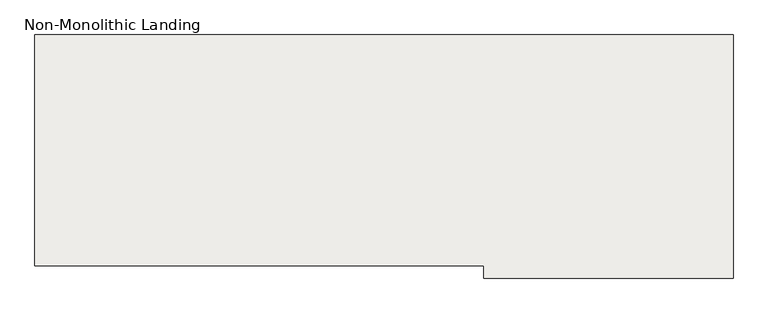
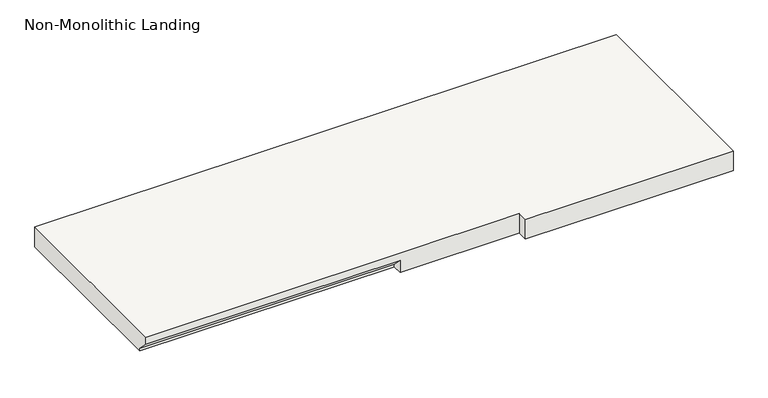
"""IFC4 building model written with IfcOpenShell, lengths in millimetres: slab geometry, Non-Monolithic Landing."""

from ifc_helpers import new_model, si_unit, origin, place, context, project, spatial, faceted_brep, source, transform, mapped, element, save


def non_monolithic_landing_1ef36e8a(model_context):
    return source(origin(), model_context, "Body", "Brep", [
        faceted_brep([(-1534.6629117, -2802.9424149, 1166.2833333), (-1534.6629117, -2777.5424149, 1140.8833333), (-912.3629117, -2777.5424149, 1140.8833333), (-912.3629117, -2802.9424149, 1166.2833333), (-620.2629117, -2802.9424149, 1185.3333333), (-620.2629117, -2828.3424149, 1185.3333333), (-112.2629117, -2828.3424149, 1185.3333333), (-112.2629117, -2802.9424149, 1185.3333333), (-112.2629117, -2333.0424149, 1185.3333333), (-1534.6629117, -2333.0424149, 1185.3333333), (-1534.6629117, -2802.9424149, 1185.3333333), (-912.3629117, -2777.5424149, 1134.5333333), (-1534.6629117, -2777.5424149, 1134.5333333), (-1534.6629117, -2333.0424149, 1134.5333333), (-112.2629117, -2333.0424149, 1134.5333333), (-112.2629117, -2802.9424149, 1134.5333333), (-112.2629117, -2828.3424149, 1134.5333333), (-620.2629117, -2828.3424149, 1134.5333333), (-620.2629117, -2802.9424149, 1134.5333333), (-912.3629117, -2802.9424149, 1134.5333333)], [[[0, 1, 2, 3]], [[4, 5, 6, 7, 8, 9, 10]], [[11, 12, 13, 14, 15, 16, 17, 18, 19]], [[12, 11, 2, 1]], [[11, 19, 3, 2]], [[4, 10, 0, 3, 19, 18]], [[5, 4, 18, 17]], [[6, 5, 17, 16]], [[7, 6, 16, 15]], [[8, 7, 15, 14]], [[9, 8, 14, 13]], [[10, 9, 13, 12, 1, 0]]]),
    ])


if __name__ == "__main__":
    model = new_model("IFC4")
    model_context = context("Model", 3, world=origin())
    ifc_project = project(units=[si_unit("LENGTHUNIT", "METRE", prefix="MILLI")], contexts=[model_context])
    site = spatial("IfcSite", under=ifc_project)
    building = spatial("IfcBuilding", under=site)
    placement = place(None, origin())
    non_monolithic_landing_shape = non_monolithic_landing_1ef36e8a(model_context)
    element("IfcSlab", 1, ObjectType="Non-Monolithic Landing", at=placement, inside=building, context=model_context, shape_type="MappedRepresentation", body=[
        mapped(non_monolithic_landing_shape, transform((0.0, 0.0, 0.0), x_axis=(1.0, 0.0, 0.0), y_axis=(0.0, 1.0, 0.0), z_axis=(0.0, 0.0, 1.0))),
    ])
    save(model, "model.ifc")
